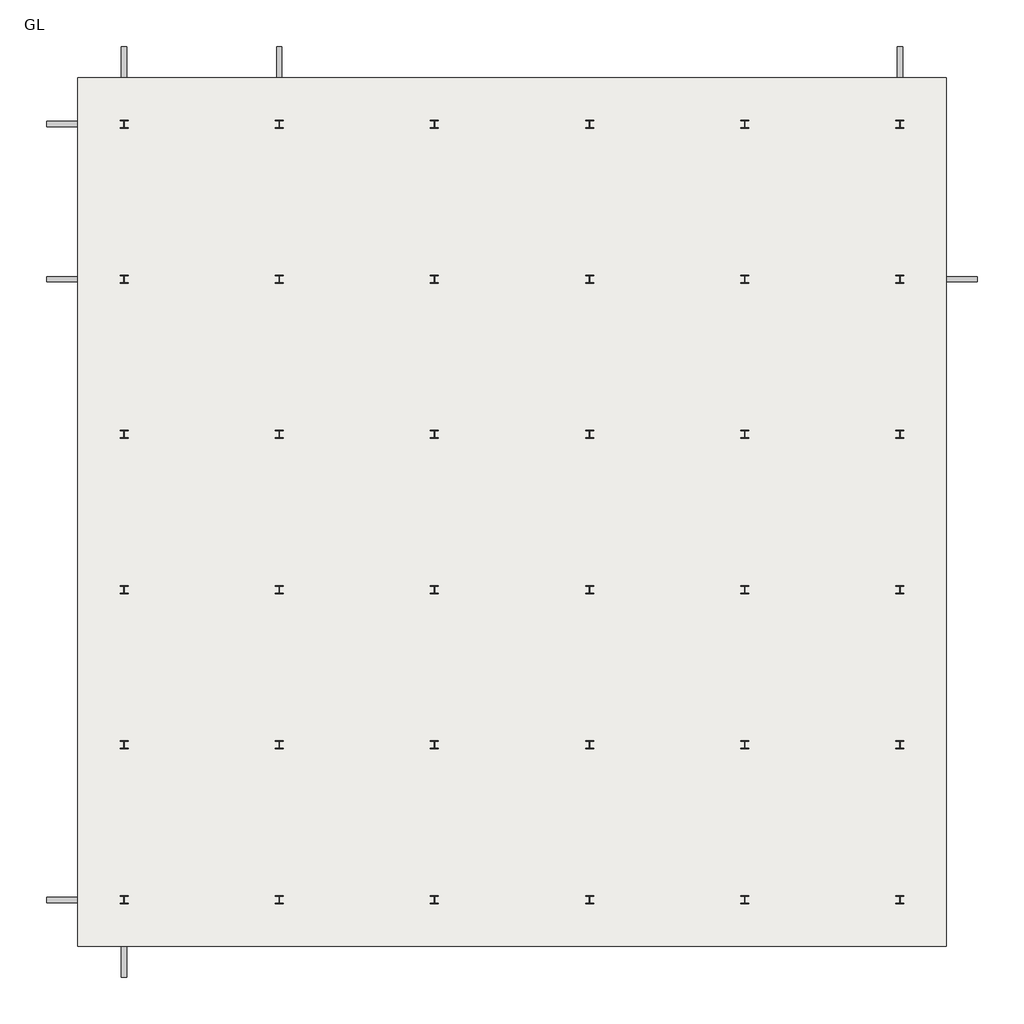
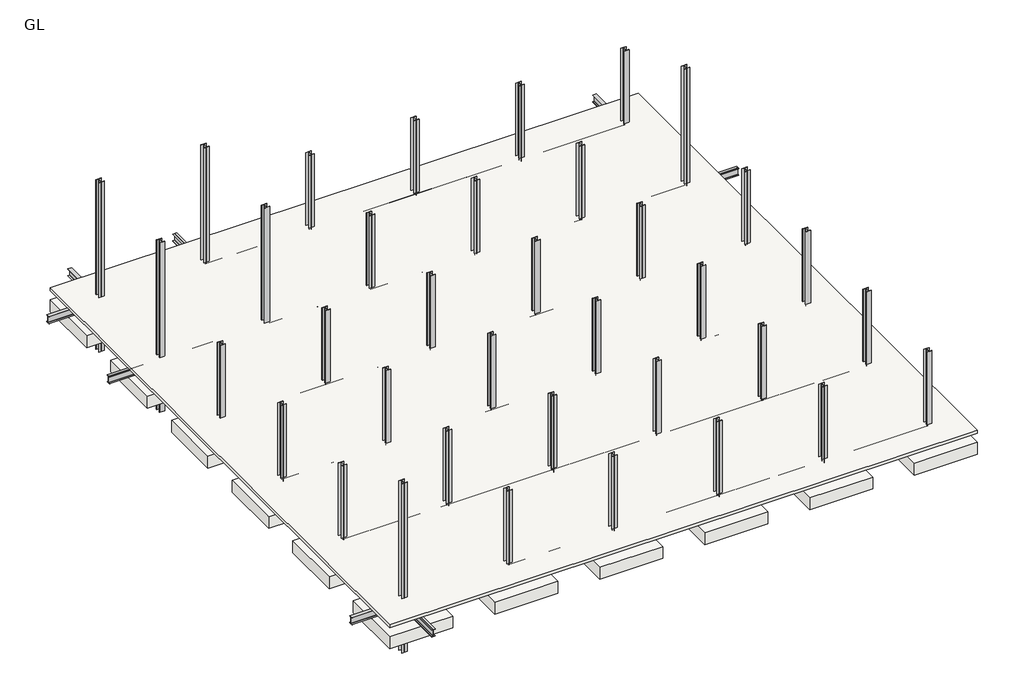
# One storey: 60 beams, 37 slabs, 36 columns.
"""IFC4 building model written with IfcOpenShell, lengths in millimetres."""

from ifc_helpers import new_model, si_unit, frame, origin, place, context, project, spatial, polyline, outline, extrude, transform, mapped, element, save
from components import w_shapes_w14x30_541e514d, w_shapes_w14x30_920474df, w_shapes_column_w10x49_053c6d64, w_shapes_column_w10x49_3bdde7d6, footing_rectangular_3mx3mx0_6m_b12d3fe5

model = new_model("IFC4")

# Units and contexts
model_context = context("Model", 3, world=origin())
ifc_project = project(units=[si_unit("LENGTHUNIT", "METRE", prefix="MILLI")], contexts=[model_context])

# Site, building, storey
site = spatial("IfcSite", under=ifc_project)
building = spatial("IfcBuilding", under=site)
storey = spatial("IfcBuildingStorey", under=building, Name="GL", Elevation=0.0)

# Beams
placement = place(None, origin())
w_shapes_w14x30_shape = w_shapes_w14x30_541e514d(model_context)
element("IfcBeam", 1, ObjectType="W Shapes : W14X30", at=placement, inside=storey, context=model_context, shape_type="MappedRepresentation", body=[
    mapped(w_shapes_w14x30_shape, transform((-15925.6378857, -5961.1374521, 281.94), x_axis=(1.0, 0.0, 0.0), y_axis=(0.0, 1.0, 0.0), z_axis=(0.0, 0.0, 1.0))),
])
element("IfcBeam", 2, ObjectType="W Shapes : W14X30", at=placement, inside=storey, context=model_context, shape_type="MappedRepresentation", body=[
    mapped(w_shapes_w14x30_shape, transform((-15925.6378857, 14038.8625479, 281.94), x_axis=(1.0, 0.0, 0.0), y_axis=(0.0, 1.0, 0.0), z_axis=(0.0, 0.0, 1.0))),
])
element("IfcBeam", 3, ObjectType="W Shapes : W14X30", at=placement, inside=storey, context=model_context, shape_type="MappedRepresentation", body=[
    mapped(w_shapes_w14x30_shape, transform((4074.3621143, 14038.8625479, 281.94), x_axis=(1.0, 0.0, 0.0), y_axis=(0.0, 1.0, 0.0), z_axis=(0.0, 0.0, 1.0))),
])
element("IfcBeam", 4, ObjectType="W Shapes : W14X30", at=placement, inside=storey, context=model_context, shape_type="MappedRepresentation", body=[
    mapped(w_shapes_w14x30_shape, transform((-15925.6378857, 19038.8625479, 281.94), x_axis=(1.0, 0.0, 0.0), y_axis=(0.0, 1.0, 0.0), z_axis=(0.0, 0.0, 1.0))),
])
element("IfcBeam", 5, ObjectType="W Shapes : W14X30", at=placement, inside=storey, context=model_context, shape_type="MappedRepresentation", body=[
    mapped(w_shapes_w14x30_shape, transform((6574.3621143, 11538.8625479, 281.94), x_axis=(0.0, 1.0, 0.0), y_axis=(-1.0, 0.0, 0.0), z_axis=(0.0, 0.0, 1.0))),
])
element("IfcBeam", 6, ObjectType="W Shapes : W14X30", at=placement, inside=storey, context=model_context, shape_type="MappedRepresentation", body=[
    mapped(w_shapes_w14x30_shape, transform((6574.3621143, 16538.8625479, 281.94), x_axis=(0.0, 1.0, 0.0), y_axis=(-1.0, 0.0, 0.0), z_axis=(0.0, 0.0, 1.0))),
])
element("IfcBeam", 7, ObjectType="W Shapes : W14X30", at=placement, inside=storey, context=model_context, shape_type="MappedRepresentation", body=[
    mapped(w_shapes_w14x30_shape, transform((-13425.6378857, 11538.8625479, 281.94), x_axis=(0.0, 1.0, 0.0), y_axis=(-1.0, 0.0, 0.0), z_axis=(0.0, 0.0, 1.0))),
])
element("IfcBeam", 8, ObjectType="W Shapes : W14X30", at=placement, inside=storey, context=model_context, shape_type="MappedRepresentation", body=[
    mapped(w_shapes_w14x30_shape, transform((-13425.6378857, 16538.8625479, 281.94), x_axis=(0.0, 1.0, 0.0), y_axis=(-1.0, 0.0, 0.0), z_axis=(0.0, 0.0, 1.0))),
])
element("IfcBeam", 9, ObjectType="W Shapes : W14X30", at=placement, inside=storey, context=model_context, shape_type="MappedRepresentation", body=[
    mapped(w_shapes_w14x30_shape, transform((-18425.6378857, -3461.1374521, 281.94), x_axis=(0.0, 1.0, 0.0), y_axis=(-1.0, 0.0, 0.0), z_axis=(0.0, 0.0, 1.0))),
])
element("IfcBeam", 10, ObjectType="W Shapes : W14X30", at=placement, inside=storey, context=model_context, shape_type="MappedRepresentation", body=[
    mapped(w_shapes_w14x30_shape, transform((-18425.6378857, 16538.8625479, 281.94), x_axis=(0.0, 1.0, 0.0), y_axis=(-1.0, 0.0, 0.0), z_axis=(0.0, 0.0, 1.0))),
])
element("IfcBeam", 11, ObjectType="W Shapes : W14X30", at=placement, inside=storey, context=model_context, shape_type="MappedRepresentation", body=[
    mapped(w_shapes_w14x30_shape, transform((-10925.6378857, 14038.8625479, 281.94), x_axis=(1.0, 0.0, 0.0), y_axis=(0.0, 1.0, 0.0), z_axis=(0.0, 0.0, 1.0))),
])
w_shapes_w14x30_2_shape = w_shapes_w14x30_920474df(model_context)
element("IfcBeam", 12, ObjectType="W Shapes : W14X30", at=placement, inside=storey, context=model_context, shape_type="MappedRepresentation", body=[
    mapped(w_shapes_w14x30_2_shape, transform((-10925.6378857, -5961.1374521, 281.94), x_axis=(1.0, 0.0, 0.0), y_axis=(0.0, 1.0, 0.0), z_axis=(0.0, 0.0, 1.0))),
])
element("IfcBeam", 13, ObjectType="W Shapes : W14X30", at=placement, inside=storey, context=model_context, shape_type="MappedRepresentation", body=[
    mapped(w_shapes_w14x30_2_shape, transform((-5925.6378857, -5961.1374521, 281.94), x_axis=(1.0, 0.0, 0.0), y_axis=(0.0, 1.0, 0.0), z_axis=(0.0, 0.0, 1.0))),
])
element("IfcBeam", 14, ObjectType="W Shapes : W14X30", at=placement, inside=storey, context=model_context, shape_type="MappedRepresentation", body=[
    mapped(w_shapes_w14x30_2_shape, transform((-925.6378857, -5961.1374521, 281.94), x_axis=(1.0, 0.0, 0.0), y_axis=(0.0, 1.0, 0.0), z_axis=(0.0, 0.0, 1.0))),
])
element("IfcBeam", 15, ObjectType="W Shapes : W14X30", at=placement, inside=storey, context=model_context, shape_type="MappedRepresentation", body=[
    mapped(w_shapes_w14x30_2_shape, transform((4074.3621143, -5961.1374521, 281.94), x_axis=(1.0, 0.0, 0.0), y_axis=(0.0, 1.0, 0.0), z_axis=(0.0, 0.0, 1.0))),
])
element("IfcBeam", 16, ObjectType="W Shapes : W14X30", at=placement, inside=storey, context=model_context, shape_type="MappedRepresentation", body=[
    mapped(w_shapes_w14x30_2_shape, transform((-15925.6378857, -961.1374521, 281.94), x_axis=(1.0, 0.0, 0.0), y_axis=(0.0, 1.0, 0.0), z_axis=(0.0, 0.0, 1.0))),
])
element("IfcBeam", 17, ObjectType="W Shapes : W14X30", at=placement, inside=storey, context=model_context, shape_type="MappedRepresentation", body=[
    mapped(w_shapes_w14x30_2_shape, transform((-10925.6378857, -961.1374521, 281.94), x_axis=(1.0, 0.0, 0.0), y_axis=(0.0, 1.0, 0.0), z_axis=(0.0, 0.0, 1.0))),
])
element("IfcBeam", 18, ObjectType="W Shapes : W14X30", at=placement, inside=storey, context=model_context, shape_type="MappedRepresentation", body=[
    mapped(w_shapes_w14x30_2_shape, transform((-5925.6378857, -961.1374521, 281.94), x_axis=(1.0, 0.0, 0.0), y_axis=(0.0, 1.0, 0.0), z_axis=(0.0, 0.0, 1.0))),
])
element("IfcBeam", 19, ObjectType="W Shapes : W14X30", at=placement, inside=storey, context=model_context, shape_type="MappedRepresentation", body=[
    mapped(w_shapes_w14x30_2_shape, transform((-925.6378857, -961.1374521, 281.94), x_axis=(1.0, 0.0, 0.0), y_axis=(0.0, 1.0, 0.0), z_axis=(0.0, 0.0, 1.0))),
])
element("IfcBeam", 20, ObjectType="W Shapes : W14X30", at=placement, inside=storey, context=model_context, shape_type="MappedRepresentation", body=[
    mapped(w_shapes_w14x30_2_shape, transform((4074.3621143, -961.1374521, 281.94), x_axis=(1.0, 0.0, 0.0), y_axis=(0.0, 1.0, 0.0), z_axis=(0.0, 0.0, 1.0))),
])
element("IfcBeam", 21, ObjectType="W Shapes : W14X30", at=placement, inside=storey, context=model_context, shape_type="MappedRepresentation", body=[
    mapped(w_shapes_w14x30_2_shape, transform((-15925.6378857, 4038.8625479, 281.94), x_axis=(1.0, 0.0, 0.0), y_axis=(0.0, 1.0, 0.0), z_axis=(0.0, 0.0, 1.0))),
])
element("IfcBeam", 22, ObjectType="W Shapes : W14X30", at=placement, inside=storey, context=model_context, shape_type="MappedRepresentation", body=[
    mapped(w_shapes_w14x30_2_shape, transform((-10925.6378857, 4038.8625479, 281.94), x_axis=(1.0, 0.0, 0.0), y_axis=(0.0, 1.0, 0.0), z_axis=(0.0, 0.0, 1.0))),
])
element("IfcBeam", 23, ObjectType="W Shapes : W14X30", at=placement, inside=storey, context=model_context, shape_type="MappedRepresentation", body=[
    mapped(w_shapes_w14x30_2_shape, transform((-5925.6378857, 4038.8625479, 281.94), x_axis=(1.0, 0.0, 0.0), y_axis=(0.0, 1.0, 0.0), z_axis=(0.0, 0.0, 1.0))),
])
element("IfcBeam", 24, ObjectType="W Shapes : W14X30", at=placement, inside=storey, context=model_context, shape_type="MappedRepresentation", body=[
    mapped(w_shapes_w14x30_2_shape, transform((-925.6378857, 4038.8625479, 281.94), x_axis=(1.0, 0.0, 0.0), y_axis=(0.0, 1.0, 0.0), z_axis=(0.0, 0.0, 1.0))),
])
element("IfcBeam", 25, ObjectType="W Shapes : W14X30", at=placement, inside=storey, context=model_context, shape_type="MappedRepresentation", body=[
    mapped(w_shapes_w14x30_2_shape, transform((4074.3621143, 4038.8625479, 281.94), x_axis=(1.0, 0.0, 0.0), y_axis=(0.0, 1.0, 0.0), z_axis=(0.0, 0.0, 1.0))),
])
element("IfcBeam", 26, ObjectType="W Shapes : W14X30", at=placement, inside=storey, context=model_context, shape_type="MappedRepresentation", body=[
    mapped(w_shapes_w14x30_2_shape, transform((-15925.6378857, 9038.8625479, 281.94), x_axis=(1.0, 0.0, 0.0), y_axis=(0.0, 1.0, 0.0), z_axis=(0.0, 0.0, 1.0))),
])
element("IfcBeam", 27, ObjectType="W Shapes : W14X30", at=placement, inside=storey, context=model_context, shape_type="MappedRepresentation", body=[
    mapped(w_shapes_w14x30_2_shape, transform((-10925.6378857, 9038.8625479, 281.94), x_axis=(1.0, 0.0, 0.0), y_axis=(0.0, 1.0, 0.0), z_axis=(0.0, 0.0, 1.0))),
])
element("IfcBeam", 28, ObjectType="W Shapes : W14X30", at=placement, inside=storey, context=model_context, shape_type="MappedRepresentation", body=[
    mapped(w_shapes_w14x30_2_shape, transform((-5925.6378857, 9038.8625479, 281.94), x_axis=(1.0, 0.0, 0.0), y_axis=(0.0, 1.0, 0.0), z_axis=(0.0, 0.0, 1.0))),
])
element("IfcBeam", 29, ObjectType="W Shapes : W14X30", at=placement, inside=storey, context=model_context, shape_type="MappedRepresentation", body=[
    mapped(w_shapes_w14x30_2_shape, transform((-925.6378857, 9038.8625479, 281.94), x_axis=(1.0, 0.0, 0.0), y_axis=(0.0, 1.0, 0.0), z_axis=(0.0, 0.0, 1.0))),
])
element("IfcBeam", 30, ObjectType="W Shapes : W14X30", at=placement, inside=storey, context=model_context, shape_type="MappedRepresentation", body=[
    mapped(w_shapes_w14x30_2_shape, transform((4074.3621143, 9038.8625479, 281.94), x_axis=(1.0, 0.0, 0.0), y_axis=(0.0, 1.0, 0.0), z_axis=(0.0, 0.0, 1.0))),
])
element("IfcBeam", 31, ObjectType="W Shapes : W14X30", at=placement, inside=storey, context=model_context, shape_type="MappedRepresentation", body=[
    mapped(w_shapes_w14x30_2_shape, transform((-5925.6378857, 14038.8625479, 281.94), x_axis=(1.0, 0.0, 0.0), y_axis=(0.0, 1.0, 0.0), z_axis=(0.0, 0.0, 1.0))),
])
element("IfcBeam", 32, ObjectType="W Shapes : W14X30", at=placement, inside=storey, context=model_context, shape_type="MappedRepresentation", body=[
    mapped(w_shapes_w14x30_2_shape, transform((-925.6378857, 14038.8625479, 281.94), x_axis=(1.0, 0.0, 0.0), y_axis=(0.0, 1.0, 0.0), z_axis=(0.0, 0.0, 1.0))),
])
element("IfcBeam", 33, ObjectType="W Shapes : W14X30", at=placement, inside=storey, context=model_context, shape_type="MappedRepresentation", body=[
    mapped(w_shapes_w14x30_2_shape, transform((-10925.6378857, 19038.8625479, 281.94), x_axis=(1.0, 0.0, 0.0), y_axis=(0.0, 1.0, 0.0), z_axis=(0.0, 0.0, 1.0))),
])
element("IfcBeam", 34, ObjectType="W Shapes : W14X30", at=placement, inside=storey, context=model_context, shape_type="MappedRepresentation", body=[
    mapped(w_shapes_w14x30_2_shape, transform((-5925.6378857, 19038.8625479, 281.94), x_axis=(1.0, 0.0, 0.0), y_axis=(0.0, 1.0, 0.0), z_axis=(0.0, 0.0, 1.0))),
])
element("IfcBeam", 35, ObjectType="W Shapes : W14X30", at=placement, inside=storey, context=model_context, shape_type="MappedRepresentation", body=[
    mapped(w_shapes_w14x30_2_shape, transform((-925.6378857, 19038.8625479, 281.94), x_axis=(1.0, 0.0, 0.0), y_axis=(0.0, 1.0, 0.0), z_axis=(0.0, 0.0, 1.0))),
])
element("IfcBeam", 36, ObjectType="W Shapes : W14X30", at=placement, inside=storey, context=model_context, shape_type="MappedRepresentation", body=[
    mapped(w_shapes_w14x30_2_shape, transform((4074.3621143, 19038.8625479, 281.94), x_axis=(1.0, 0.0, 0.0), y_axis=(0.0, 1.0, 0.0), z_axis=(0.0, 0.0, 1.0))),
])
element("IfcBeam", 37, ObjectType="W Shapes : W14X30", at=placement, inside=storey, context=model_context, shape_type="MappedRepresentation", body=[
    mapped(w_shapes_w14x30_2_shape, transform((6574.3621143, -3461.1374521, 281.94), x_axis=(0.0, 1.0, 0.0), y_axis=(-1.0, 0.0, 0.0), z_axis=(0.0, 0.0, 1.0))),
])
element("IfcBeam", 38, ObjectType="W Shapes : W14X30", at=placement, inside=storey, context=model_context, shape_type="MappedRepresentation", body=[
    mapped(w_shapes_w14x30_2_shape, transform((6574.3621143, 1538.8625479, 281.94), x_axis=(0.0, 1.0, 0.0), y_axis=(-1.0, 0.0, 0.0), z_axis=(0.0, 0.0, 1.0))),
])
element("IfcBeam", 39, ObjectType="W Shapes : W14X30", at=placement, inside=storey, context=model_context, shape_type="MappedRepresentation", body=[
    mapped(w_shapes_w14x30_2_shape, transform((6574.3621143, 6538.8625479, 281.94), x_axis=(0.0, 1.0, 0.0), y_axis=(-1.0, 0.0, 0.0), z_axis=(0.0, 0.0, 1.0))),
])
element("IfcBeam", 40, ObjectType="W Shapes : W14X30", at=placement, inside=storey, context=model_context, shape_type="MappedRepresentation", body=[
    mapped(w_shapes_w14x30_2_shape, transform((1574.3621143, -3461.1374521, 281.94), x_axis=(0.0, 1.0, 0.0), y_axis=(-1.0, 0.0, 0.0), z_axis=(0.0, 0.0, 1.0))),
])
element("IfcBeam", 41, ObjectType="W Shapes : W14X30", at=placement, inside=storey, context=model_context, shape_type="MappedRepresentation", body=[
    mapped(w_shapes_w14x30_2_shape, transform((1574.3621143, 1538.8625479, 281.94), x_axis=(0.0, 1.0, 0.0), y_axis=(-1.0, 0.0, 0.0), z_axis=(0.0, 0.0, 1.0))),
])
element("IfcBeam", 42, ObjectType="W Shapes : W14X30", at=placement, inside=storey, context=model_context, shape_type="MappedRepresentation", body=[
    mapped(w_shapes_w14x30_2_shape, transform((1574.3621143, 6538.8625479, 281.94), x_axis=(0.0, 1.0, 0.0), y_axis=(-1.0, 0.0, 0.0), z_axis=(0.0, 0.0, 1.0))),
])
element("IfcBeam", 43, ObjectType="W Shapes : W14X30", at=placement, inside=storey, context=model_context, shape_type="MappedRepresentation", body=[
    mapped(w_shapes_w14x30_2_shape, transform((1574.3621143, 11538.8625479, 281.94), x_axis=(0.0, 1.0, 0.0), y_axis=(-1.0, 0.0, 0.0), z_axis=(0.0, 0.0, 1.0))),
])
element("IfcBeam", 44, ObjectType="W Shapes : W14X30", at=placement, inside=storey, context=model_context, shape_type="MappedRepresentation", body=[
    mapped(w_shapes_w14x30_2_shape, transform((1574.3621143, 16538.8625479, 281.94), x_axis=(0.0, 1.0, 0.0), y_axis=(-1.0, 0.0, 0.0), z_axis=(0.0, 0.0, 1.0))),
])
element("IfcBeam", 45, ObjectType="W Shapes : W14X30", at=placement, inside=storey, context=model_context, shape_type="MappedRepresentation", body=[
    mapped(w_shapes_w14x30_2_shape, transform((-3425.6378857, -3461.1374521, 281.94), x_axis=(0.0, 1.0, 0.0), y_axis=(-1.0, 0.0, 0.0), z_axis=(0.0, 0.0, 1.0))),
])
element("IfcBeam", 46, ObjectType="W Shapes : W14X30", at=placement, inside=storey, context=model_context, shape_type="MappedRepresentation", body=[
    mapped(w_shapes_w14x30_2_shape, transform((-3425.6378857, 1538.8625479, 281.94), x_axis=(0.0, 1.0, 0.0), y_axis=(-1.0, 0.0, 0.0), z_axis=(0.0, 0.0, 1.0))),
])
element("IfcBeam", 47, ObjectType="W Shapes : W14X30", at=placement, inside=storey, context=model_context, shape_type="MappedRepresentation", body=[
    mapped(w_shapes_w14x30_2_shape, transform((-3425.6378857, 6538.8625479, 281.94), x_axis=(0.0, 1.0, 0.0), y_axis=(-1.0, 0.0, 0.0), z_axis=(0.0, 0.0, 1.0))),
])
element("IfcBeam", 48, ObjectType="W Shapes : W14X30", at=placement, inside=storey, context=model_context, shape_type="MappedRepresentation", body=[
    mapped(w_shapes_w14x30_2_shape, transform((-3425.6378857, 11538.8625479, 281.94), x_axis=(0.0, 1.0, 0.0), y_axis=(-1.0, 0.0, 0.0), z_axis=(0.0, 0.0, 1.0))),
])
element("IfcBeam", 49, ObjectType="W Shapes : W14X30", at=placement, inside=storey, context=model_context, shape_type="MappedRepresentation", body=[
    mapped(w_shapes_w14x30_2_shape, transform((-3425.6378857, 16538.8625479, 281.94), x_axis=(0.0, 1.0, 0.0), y_axis=(-1.0, 0.0, 0.0), z_axis=(0.0, 0.0, 1.0))),
])
element("IfcBeam", 50, ObjectType="W Shapes : W14X30", at=placement, inside=storey, context=model_context, shape_type="MappedRepresentation", body=[
    mapped(w_shapes_w14x30_2_shape, transform((-8425.6378857, -3461.1374521, 281.94), x_axis=(0.0, 1.0, 0.0), y_axis=(-1.0, 0.0, 0.0), z_axis=(0.0, 0.0, 1.0))),
])
element("IfcBeam", 51, ObjectType="W Shapes : W14X30", at=placement, inside=storey, context=model_context, shape_type="MappedRepresentation", body=[
    mapped(w_shapes_w14x30_2_shape, transform((-8425.6378857, 1538.8625479, 281.94), x_axis=(0.0, 1.0, 0.0), y_axis=(-1.0, 0.0, 0.0), z_axis=(0.0, 0.0, 1.0))),
])
element("IfcBeam", 52, ObjectType="W Shapes : W14X30", at=placement, inside=storey, context=model_context, shape_type="MappedRepresentation", body=[
    mapped(w_shapes_w14x30_2_shape, transform((-8425.6378857, 6538.8625479, 281.94), x_axis=(0.0, 1.0, 0.0), y_axis=(-1.0, 0.0, 0.0), z_axis=(0.0, 0.0, 1.0))),
])
element("IfcBeam", 53, ObjectType="W Shapes : W14X30", at=placement, inside=storey, context=model_context, shape_type="MappedRepresentation", body=[
    mapped(w_shapes_w14x30_2_shape, transform((-8425.6378857, 11538.8625479, 281.94), x_axis=(0.0, 1.0, 0.0), y_axis=(-1.0, 0.0, 0.0), z_axis=(0.0, 0.0, 1.0))),
])
element("IfcBeam", 54, ObjectType="W Shapes : W14X30", at=placement, inside=storey, context=model_context, shape_type="MappedRepresentation", body=[
    mapped(w_shapes_w14x30_2_shape, transform((-8425.6378857, 16538.8625479, 281.94), x_axis=(0.0, 1.0, 0.0), y_axis=(-1.0, 0.0, 0.0), z_axis=(0.0, 0.0, 1.0))),
])
element("IfcBeam", 55, ObjectType="W Shapes : W14X30", at=placement, inside=storey, context=model_context, shape_type="MappedRepresentation", body=[
    mapped(w_shapes_w14x30_2_shape, transform((-13425.6378857, -3461.1374521, 281.94), x_axis=(0.0, 1.0, 0.0), y_axis=(-1.0, 0.0, 0.0), z_axis=(0.0, 0.0, 1.0))),
])
element("IfcBeam", 56, ObjectType="W Shapes : W14X30", at=placement, inside=storey, context=model_context, shape_type="MappedRepresentation", body=[
    mapped(w_shapes_w14x30_2_shape, transform((-13425.6378857, 1538.8625479, 281.94), x_axis=(0.0, 1.0, 0.0), y_axis=(-1.0, 0.0, 0.0), z_axis=(0.0, 0.0, 1.0))),
])
element("IfcBeam", 57, ObjectType="W Shapes : W14X30", at=placement, inside=storey, context=model_context, shape_type="MappedRepresentation", body=[
    mapped(w_shapes_w14x30_2_shape, transform((-13425.6378857, 6538.8625479, 281.94), x_axis=(0.0, 1.0, 0.0), y_axis=(-1.0, 0.0, 0.0), z_axis=(0.0, 0.0, 1.0))),
])
element("IfcBeam", 58, ObjectType="W Shapes : W14X30", at=placement, inside=storey, context=model_context, shape_type="MappedRepresentation", body=[
    mapped(w_shapes_w14x30_2_shape, transform((-18425.6378857, 1538.8625479, 281.94), x_axis=(0.0, 1.0, 0.0), y_axis=(-1.0, 0.0, 0.0), z_axis=(0.0, 0.0, 1.0))),
])
element("IfcBeam", 59, ObjectType="W Shapes : W14X30", at=placement, inside=storey, context=model_context, shape_type="MappedRepresentation", body=[
    mapped(w_shapes_w14x30_2_shape, transform((-18425.6378857, 6538.8625479, 281.94), x_axis=(0.0, 1.0, 0.0), y_axis=(-1.0, 0.0, 0.0), z_axis=(0.0, 0.0, 1.0))),
])
element("IfcBeam", 60, ObjectType="W Shapes : W14X30", at=placement, inside=storey, context=model_context, shape_type="MappedRepresentation", body=[
    mapped(w_shapes_w14x30_2_shape, transform((-18425.6378857, 11538.8625479, 281.94), x_axis=(0.0, 1.0, 0.0), y_axis=(-1.0, 0.0, 0.0), z_axis=(0.0, 0.0, 1.0))),
])

# Columns
w_shapes_column_w10x49_shape = w_shapes_column_w10x49_053c6d64(model_context)
element("IfcColumn", 61, ObjectType="W Shapes-Column : W10X49", at=placement, inside=storey, context=model_context, shape_type="MappedRepresentation", body=[
    mapped(w_shapes_column_w10x49_shape, transform((6574.3621143, -5961.1374521, 0.0), x_axis=(1.0, 0.0, 0.0), y_axis=(0.0, 1.0, 0.0), z_axis=(0.0, 0.0, 1.0))),
])
element("IfcColumn", 62, ObjectType="W Shapes-Column : W10X49", at=placement, inside=storey, context=model_context, shape_type="MappedRepresentation", body=[
    mapped(w_shapes_column_w10x49_shape, transform((1574.3621143, -5961.1374521, 0.0), x_axis=(1.0, 0.0, 0.0), y_axis=(0.0, 1.0, 0.0), z_axis=(0.0, 0.0, 1.0))),
])
element("IfcColumn", 63, ObjectType="W Shapes-Column : W10X49", at=placement, inside=storey, context=model_context, shape_type="MappedRepresentation", body=[
    mapped(w_shapes_column_w10x49_shape, transform((-3425.6378857, -5961.1374521, 0.0), x_axis=(1.0, 0.0, 0.0), y_axis=(0.0, 1.0, 0.0), z_axis=(0.0, 0.0, 1.0))),
])
element("IfcColumn", 64, ObjectType="W Shapes-Column : W10X49", at=placement, inside=storey, context=model_context, shape_type="MappedRepresentation", body=[
    mapped(w_shapes_column_w10x49_shape, transform((-8425.6378857, -5961.1374521, 0.0), x_axis=(1.0, 0.0, 0.0), y_axis=(0.0, 1.0, 0.0), z_axis=(0.0, 0.0, 1.0))),
])
element("IfcColumn", 65, ObjectType="W Shapes-Column : W10X49", at=placement, inside=storey, context=model_context, shape_type="MappedRepresentation", body=[
    mapped(w_shapes_column_w10x49_shape, transform((-13425.6378857, -5961.1374521, 0.0), x_axis=(1.0, 0.0, 0.0), y_axis=(0.0, 1.0, 0.0), z_axis=(0.0, 0.0, 1.0))),
])
element("IfcColumn", 66, ObjectType="W Shapes-Column : W10X49", at=placement, inside=storey, context=model_context, shape_type="MappedRepresentation", body=[
    mapped(w_shapes_column_w10x49_shape, transform((6574.3621143, -961.1374521, 0.0), x_axis=(1.0, 0.0, 0.0), y_axis=(0.0, 1.0, 0.0), z_axis=(0.0, 0.0, 1.0))),
])
element("IfcColumn", 67, ObjectType="W Shapes-Column : W10X49", at=placement, inside=storey, context=model_context, shape_type="MappedRepresentation", body=[
    mapped(w_shapes_column_w10x49_shape, transform((1574.3621143, -961.1374521, 0.0), x_axis=(1.0, 0.0, 0.0), y_axis=(0.0, 1.0, 0.0), z_axis=(0.0, 0.0, 1.0))),
])
element("IfcColumn", 68, ObjectType="W Shapes-Column : W10X49", at=placement, inside=storey, context=model_context, shape_type="MappedRepresentation", body=[
    mapped(w_shapes_column_w10x49_shape, transform((-3425.6378857, -961.1374521, 0.0), x_axis=(1.0, 0.0, 0.0), y_axis=(0.0, 1.0, 0.0), z_axis=(0.0, 0.0, 1.0))),
])
element("IfcColumn", 69, ObjectType="W Shapes-Column : W10X49", at=placement, inside=storey, context=model_context, shape_type="MappedRepresentation", body=[
    mapped(w_shapes_column_w10x49_shape, transform((-8425.6378857, -961.1374521, 0.0), x_axis=(1.0, 0.0, 0.0), y_axis=(0.0, 1.0, 0.0), z_axis=(0.0, 0.0, 1.0))),
])
element("IfcColumn", 70, ObjectType="W Shapes-Column : W10X49", at=placement, inside=storey, context=model_context, shape_type="MappedRepresentation", body=[
    mapped(w_shapes_column_w10x49_shape, transform((-13425.6378857, -961.1374521, 0.0), x_axis=(1.0, 0.0, 0.0), y_axis=(0.0, 1.0, 0.0), z_axis=(0.0, 0.0, 1.0))),
])
element("IfcColumn", 71, ObjectType="W Shapes-Column : W10X49", at=placement, inside=storey, context=model_context, shape_type="MappedRepresentation", body=[
    mapped(w_shapes_column_w10x49_shape, transform((-18425.6378857, -961.1374521, 0.0), x_axis=(1.0, 0.0, 0.0), y_axis=(0.0, 1.0, 0.0), z_axis=(0.0, 0.0, 1.0))),
])
element("IfcColumn", 72, ObjectType="W Shapes-Column : W10X49", at=placement, inside=storey, context=model_context, shape_type="MappedRepresentation", body=[
    mapped(w_shapes_column_w10x49_shape, transform((6574.3621143, 4038.8625479, 0.0), x_axis=(1.0, 0.0, 0.0), y_axis=(0.0, 1.0, 0.0), z_axis=(0.0, 0.0, 1.0))),
])
element("IfcColumn", 73, ObjectType="W Shapes-Column : W10X49", at=placement, inside=storey, context=model_context, shape_type="MappedRepresentation", body=[
    mapped(w_shapes_column_w10x49_shape, transform((1574.3621143, 4038.8625479, 0.0), x_axis=(1.0, 0.0, 0.0), y_axis=(0.0, 1.0, 0.0), z_axis=(0.0, 0.0, 1.0))),
])
element("IfcColumn", 74, ObjectType="W Shapes-Column : W10X49", at=placement, inside=storey, context=model_context, shape_type="MappedRepresentation", body=[
    mapped(w_shapes_column_w10x49_shape, transform((-3425.6378857, 4038.8625479, 0.0), x_axis=(1.0, 0.0, 0.0), y_axis=(0.0, 1.0, 0.0), z_axis=(0.0, 0.0, 1.0))),
])
element("IfcColumn", 75, ObjectType="W Shapes-Column : W10X49", at=placement, inside=storey, context=model_context, shape_type="MappedRepresentation", body=[
    mapped(w_shapes_column_w10x49_shape, transform((-8425.6378857, 4038.8625479, 0.0), x_axis=(1.0, 0.0, 0.0), y_axis=(0.0, 1.0, 0.0), z_axis=(0.0, 0.0, 1.0))),
])
element("IfcColumn", 76, ObjectType="W Shapes-Column : W10X49", at=placement, inside=storey, context=model_context, shape_type="MappedRepresentation", body=[
    mapped(w_shapes_column_w10x49_shape, transform((-13425.6378857, 4038.8625479, 0.0), x_axis=(1.0, 0.0, 0.0), y_axis=(0.0, 1.0, 0.0), z_axis=(0.0, 0.0, 1.0))),
])
element("IfcColumn", 77, ObjectType="W Shapes-Column : W10X49", at=placement, inside=storey, context=model_context, shape_type="MappedRepresentation", body=[
    mapped(w_shapes_column_w10x49_shape, transform((-18425.6378857, 4038.8625479, 0.0), x_axis=(1.0, 0.0, 0.0), y_axis=(0.0, 1.0, 0.0), z_axis=(0.0, 0.0, 1.0))),
])
element("IfcColumn", 78, ObjectType="W Shapes-Column : W10X49", at=placement, inside=storey, context=model_context, shape_type="MappedRepresentation", body=[
    mapped(w_shapes_column_w10x49_shape, transform((6574.3621143, 9038.8625479, 0.0), x_axis=(1.0, 0.0, 0.0), y_axis=(0.0, 1.0, 0.0), z_axis=(0.0, 0.0, 1.0))),
])
element("IfcColumn", 79, ObjectType="W Shapes-Column : W10X49", at=placement, inside=storey, context=model_context, shape_type="MappedRepresentation", body=[
    mapped(w_shapes_column_w10x49_shape, transform((1574.3621143, 9038.8625479, 0.0), x_axis=(1.0, 0.0, 0.0), y_axis=(0.0, 1.0, 0.0), z_axis=(0.0, 0.0, 1.0))),
])
element("IfcColumn", 80, ObjectType="W Shapes-Column : W10X49", at=placement, inside=storey, context=model_context, shape_type="MappedRepresentation", body=[
    mapped(w_shapes_column_w10x49_shape, transform((-3425.6378857, 9038.8625479, 0.0), x_axis=(1.0, 0.0, 0.0), y_axis=(0.0, 1.0, 0.0), z_axis=(0.0, 0.0, 1.0))),
])
element("IfcColumn", 81, ObjectType="W Shapes-Column : W10X49", at=placement, inside=storey, context=model_context, shape_type="MappedRepresentation", body=[
    mapped(w_shapes_column_w10x49_shape, transform((-8425.6378857, 9038.8625479, 0.0), x_axis=(1.0, 0.0, 0.0), y_axis=(0.0, 1.0, 0.0), z_axis=(0.0, 0.0, 1.0))),
])
element("IfcColumn", 82, ObjectType="W Shapes-Column : W10X49", at=placement, inside=storey, context=model_context, shape_type="MappedRepresentation", body=[
    mapped(w_shapes_column_w10x49_shape, transform((-13425.6378857, 9038.8625479, 0.0), x_axis=(1.0, 0.0, 0.0), y_axis=(0.0, 1.0, 0.0), z_axis=(0.0, 0.0, 1.0))),
])
element("IfcColumn", 83, ObjectType="W Shapes-Column : W10X49", at=placement, inside=storey, context=model_context, shape_type="MappedRepresentation", body=[
    mapped(w_shapes_column_w10x49_shape, transform((-18425.6378857, 9038.8625479, 0.0), x_axis=(1.0, 0.0, 0.0), y_axis=(0.0, 1.0, 0.0), z_axis=(0.0, 0.0, 1.0))),
])
element("IfcColumn", 84, ObjectType="W Shapes-Column : W10X49", at=placement, inside=storey, context=model_context, shape_type="MappedRepresentation", body=[
    mapped(w_shapes_column_w10x49_shape, transform((1574.3621143, 14038.8625479, 0.0), x_axis=(1.0, 0.0, 0.0), y_axis=(0.0, 1.0, 0.0), z_axis=(0.0, 0.0, 1.0))),
])
element("IfcColumn", 85, ObjectType="W Shapes-Column : W10X49", at=placement, inside=storey, context=model_context, shape_type="MappedRepresentation", body=[
    mapped(w_shapes_column_w10x49_shape, transform((-3425.6378857, 14038.8625479, 0.0), x_axis=(1.0, 0.0, 0.0), y_axis=(0.0, 1.0, 0.0), z_axis=(0.0, 0.0, 1.0))),
])
element("IfcColumn", 86, ObjectType="W Shapes-Column : W10X49", at=placement, inside=storey, context=model_context, shape_type="MappedRepresentation", body=[
    mapped(w_shapes_column_w10x49_shape, transform((-8425.6378857, 14038.8625479, 0.0), x_axis=(1.0, 0.0, 0.0), y_axis=(0.0, 1.0, 0.0), z_axis=(0.0, 0.0, 1.0))),
])
element("IfcColumn", 87, ObjectType="W Shapes-Column : W10X49", at=placement, inside=storey, context=model_context, shape_type="MappedRepresentation", body=[
    mapped(w_shapes_column_w10x49_shape, transform((6574.3621143, 19038.8625479, 0.0), x_axis=(1.0, 0.0, 0.0), y_axis=(0.0, 1.0, 0.0), z_axis=(0.0, 0.0, 1.0))),
])
element("IfcColumn", 88, ObjectType="W Shapes-Column : W10X49", at=placement, inside=storey, context=model_context, shape_type="MappedRepresentation", body=[
    mapped(w_shapes_column_w10x49_shape, transform((1574.3621143, 19038.8625479, 0.0), x_axis=(1.0, 0.0, 0.0), y_axis=(0.0, 1.0, 0.0), z_axis=(0.0, 0.0, 1.0))),
])
element("IfcColumn", 89, ObjectType="W Shapes-Column : W10X49", at=placement, inside=storey, context=model_context, shape_type="MappedRepresentation", body=[
    mapped(w_shapes_column_w10x49_shape, transform((-3425.6378857, 19038.8625479, 0.0), x_axis=(1.0, 0.0, 0.0), y_axis=(0.0, 1.0, 0.0), z_axis=(0.0, 0.0, 1.0))),
])
element("IfcColumn", 90, ObjectType="W Shapes-Column : W10X49", at=placement, inside=storey, context=model_context, shape_type="MappedRepresentation", body=[
    mapped(w_shapes_column_w10x49_shape, transform((-8425.6378857, 19038.8625479, 0.0), x_axis=(1.0, 0.0, 0.0), y_axis=(0.0, 1.0, 0.0), z_axis=(0.0, 0.0, 1.0))),
])
w_shapes_column_w10x49_2_shape = w_shapes_column_w10x49_3bdde7d6(model_context)
element("IfcColumn", 91, ObjectType="W Shapes-Column : W10X49", at=placement, inside=storey, context=model_context, shape_type="MappedRepresentation", body=[
    mapped(w_shapes_column_w10x49_2_shape, transform((-18425.6378857, -5961.1374521, 0.0), x_axis=(1.0, 0.0, 0.0), y_axis=(0.0, 1.0, 0.0), z_axis=(0.0, 0.0, 1.0))),
])
element("IfcColumn", 92, ObjectType="W Shapes-Column : W10X49", at=placement, inside=storey, context=model_context, shape_type="MappedRepresentation", body=[
    mapped(w_shapes_column_w10x49_2_shape, transform((6574.3621143, 14038.8625479, 0.0), x_axis=(1.0, 0.0, 0.0), y_axis=(0.0, 1.0, 0.0), z_axis=(0.0, 0.0, 1.0))),
])
element("IfcColumn", 93, ObjectType="W Shapes-Column : W10X49", at=placement, inside=storey, context=model_context, shape_type="MappedRepresentation", body=[
    mapped(w_shapes_column_w10x49_2_shape, transform((-13425.6378857, 14038.8625479, 0.0), x_axis=(1.0, 0.0, 0.0), y_axis=(0.0, 1.0, 0.0), z_axis=(0.0, 0.0, 1.0))),
])
element("IfcColumn", 94, ObjectType="W Shapes-Column : W10X49", at=placement, inside=storey, context=model_context, shape_type="MappedRepresentation", body=[
    mapped(w_shapes_column_w10x49_2_shape, transform((-18425.6378857, 14038.8625479, 0.0), x_axis=(1.0, 0.0, 0.0), y_axis=(0.0, 1.0, 0.0), z_axis=(0.0, 0.0, 1.0))),
])
element("IfcColumn", 95, ObjectType="W Shapes-Column : W10X49", at=placement, inside=storey, context=model_context, shape_type="MappedRepresentation", body=[
    mapped(w_shapes_column_w10x49_2_shape, transform((-13425.6378857, 19038.8625479, 0.0), x_axis=(1.0, 0.0, 0.0), y_axis=(0.0, 1.0, 0.0), z_axis=(0.0, 0.0, 1.0))),
])
element("IfcColumn", 96, ObjectType="W Shapes-Column : W10X49", at=placement, inside=storey, context=model_context, shape_type="MappedRepresentation", body=[
    mapped(w_shapes_column_w10x49_2_shape, transform((-18425.6378857, 19038.8625479, 0.0), x_axis=(1.0, 0.0, 0.0), y_axis=(0.0, 1.0, 0.0), z_axis=(0.0, 0.0, 1.0))),
])

# Slabs
element("IfcSlab", 97, ObjectType="6\" Concrete", at=placement, inside=storey, context=model_context, shape_type="SweptSolid", body=[
    extrude(outline(polyline([(8074.3511768, 20538.8516104), (8074.3511768, -7461.1265146), (-19925.6269482, -7461.1265146), (-19925.6269482, 20538.8516104), (8074.3511768, 20538.8516104)])), frame((0.0, 0.0, 457.2), z_axis=(0.0, 0.0, 1.0), x_axis=(1.0, 0.0, 0.0)), (0.0, 0.0, 1.0), 152.4),
])
footing_rectangular_3mx3mx0_6m_shape = footing_rectangular_3mx3mx0_6m_b12d3fe5(model_context)
element("IfcSlab", 98, ObjectType="Footing-Rectangular : 3mx3mx0.6m", at=placement, inside=storey, context=model_context, shape_type="MappedRepresentation", body=[
    mapped(footing_rectangular_3mx3mx0_6m_shape, transform((6574.3621143, -5961.1374521, 0.0), x_axis=(1.0, 0.0, 0.0), y_axis=(0.0, 1.0, 0.0), z_axis=(0.0, 0.0, 1.0))),
])
element("IfcSlab", 99, ObjectType="Footing-Rectangular : 3mx3mx0.6m", at=placement, inside=storey, context=model_context, shape_type="MappedRepresentation", body=[
    mapped(footing_rectangular_3mx3mx0_6m_shape, transform((1574.3621143, -5961.1374521, 0.0), x_axis=(1.0, 0.0, 0.0), y_axis=(0.0, 1.0, 0.0), z_axis=(0.0, 0.0, 1.0))),
])
element("IfcSlab", 100, ObjectType="Footing-Rectangular : 3mx3mx0.6m", at=placement, inside=storey, context=model_context, shape_type="MappedRepresentation", body=[
    mapped(footing_rectangular_3mx3mx0_6m_shape, transform((-3425.6378857, -5961.1374521, 0.0), x_axis=(1.0, 0.0, 0.0), y_axis=(0.0, 1.0, 0.0), z_axis=(0.0, 0.0, 1.0))),
])
element("IfcSlab", 101, ObjectType="Footing-Rectangular : 3mx3mx0.6m", at=placement, inside=storey, context=model_context, shape_type="MappedRepresentation", body=[
    mapped(footing_rectangular_3mx3mx0_6m_shape, transform((-8425.6378857, -5961.1374521, 0.0), x_axis=(1.0, 0.0, 0.0), y_axis=(0.0, 1.0, 0.0), z_axis=(0.0, 0.0, 1.0))),
])
element("IfcSlab", 102, ObjectType="Footing-Rectangular : 3mx3mx0.6m", at=placement, inside=storey, context=model_context, shape_type="MappedRepresentation", body=[
    mapped(footing_rectangular_3mx3mx0_6m_shape, transform((-13425.6378857, -5961.1374521, 0.0), x_axis=(1.0, 0.0, 0.0), y_axis=(0.0, 1.0, 0.0), z_axis=(0.0, 0.0, 1.0))),
])
element("IfcSlab", 103, ObjectType="Footing-Rectangular : 3mx3mx0.6m", at=placement, inside=storey, context=model_context, shape_type="MappedRepresentation", body=[
    mapped(footing_rectangular_3mx3mx0_6m_shape, transform((-18425.6378857, -5961.1374521, 0.0), x_axis=(1.0, 0.0, 0.0), y_axis=(0.0, 1.0, 0.0), z_axis=(0.0, 0.0, 1.0))),
])
element("IfcSlab", 104, ObjectType="Footing-Rectangular : 3mx3mx0.6m", at=placement, inside=storey, context=model_context, shape_type="MappedRepresentation", body=[
    mapped(footing_rectangular_3mx3mx0_6m_shape, transform((6574.3621143, -961.1374521, 0.0), x_axis=(1.0, 0.0, 0.0), y_axis=(0.0, 1.0, 0.0), z_axis=(0.0, 0.0, 1.0))),
])
element("IfcSlab", 105, ObjectType="Footing-Rectangular : 3mx3mx0.6m", at=placement, inside=storey, context=model_context, shape_type="MappedRepresentation", body=[
    mapped(footing_rectangular_3mx3mx0_6m_shape, transform((1574.3621143, -961.1374521, 0.0), x_axis=(1.0, 0.0, 0.0), y_axis=(0.0, 1.0, 0.0), z_axis=(0.0, 0.0, 1.0))),
])
element("IfcSlab", 106, ObjectType="Footing-Rectangular : 3mx3mx0.6m", at=placement, inside=storey, context=model_context, shape_type="MappedRepresentation", body=[
    mapped(footing_rectangular_3mx3mx0_6m_shape, transform((-3425.6378857, -961.1374521, 0.0), x_axis=(1.0, 0.0, 0.0), y_axis=(0.0, 1.0, 0.0), z_axis=(0.0, 0.0, 1.0))),
])
element("IfcSlab", 107, ObjectType="Footing-Rectangular : 3mx3mx0.6m", at=placement, inside=storey, context=model_context, shape_type="MappedRepresentation", body=[
    mapped(footing_rectangular_3mx3mx0_6m_shape, transform((-8425.6378857, -961.1374521, 0.0), x_axis=(1.0, 0.0, 0.0), y_axis=(0.0, 1.0, 0.0), z_axis=(0.0, 0.0, 1.0))),
])
element("IfcSlab", 108, ObjectType="Footing-Rectangular : 3mx3mx0.6m", at=placement, inside=storey, context=model_context, shape_type="MappedRepresentation", body=[
    mapped(footing_rectangular_3mx3mx0_6m_shape, transform((-13425.6378857, -961.1374521, 0.0), x_axis=(1.0, 0.0, 0.0), y_axis=(0.0, 1.0, 0.0), z_axis=(0.0, 0.0, 1.0))),
])
element("IfcSlab", 109, ObjectType="Footing-Rectangular : 3mx3mx0.6m", at=placement, inside=storey, context=model_context, shape_type="MappedRepresentation", body=[
    mapped(footing_rectangular_3mx3mx0_6m_shape, transform((-18425.6378857, -961.1374521, 0.0), x_axis=(1.0, 0.0, 0.0), y_axis=(0.0, 1.0, 0.0), z_axis=(0.0, 0.0, 1.0))),
])
element("IfcSlab", 110, ObjectType="Footing-Rectangular : 3mx3mx0.6m", at=placement, inside=storey, context=model_context, shape_type="MappedRepresentation", body=[
    mapped(footing_rectangular_3mx3mx0_6m_shape, transform((6574.3621143, 4038.8625479, 0.0), x_axis=(1.0, 0.0, 0.0), y_axis=(0.0, 1.0, 0.0), z_axis=(0.0, 0.0, 1.0))),
])
element("IfcSlab", 111, ObjectType="Footing-Rectangular : 3mx3mx0.6m", at=placement, inside=storey, context=model_context, shape_type="MappedRepresentation", body=[
    mapped(footing_rectangular_3mx3mx0_6m_shape, transform((1574.3621143, 4038.8625479, 0.0), x_axis=(1.0, 0.0, 0.0), y_axis=(0.0, 1.0, 0.0), z_axis=(0.0, 0.0, 1.0))),
])
element("IfcSlab", 112, ObjectType="Footing-Rectangular : 3mx3mx0.6m", at=placement, inside=storey, context=model_context, shape_type="MappedRepresentation", body=[
    mapped(footing_rectangular_3mx3mx0_6m_shape, transform((-3425.6378857, 4038.8625479, 0.0), x_axis=(1.0, 0.0, 0.0), y_axis=(0.0, 1.0, 0.0), z_axis=(0.0, 0.0, 1.0))),
])
element("IfcSlab", 113, ObjectType="Footing-Rectangular : 3mx3mx0.6m", at=placement, inside=storey, context=model_context, shape_type="MappedRepresentation", body=[
    mapped(footing_rectangular_3mx3mx0_6m_shape, transform((-8425.6378857, 4038.8625479, 0.0), x_axis=(1.0, 0.0, 0.0), y_axis=(0.0, 1.0, 0.0), z_axis=(0.0, 0.0, 1.0))),
])
element("IfcSlab", 114, ObjectType="Footing-Rectangular : 3mx3mx0.6m", at=placement, inside=storey, context=model_context, shape_type="MappedRepresentation", body=[
    mapped(footing_rectangular_3mx3mx0_6m_shape, transform((-13425.6378857, 4038.8625479, 0.0), x_axis=(1.0, 0.0, 0.0), y_axis=(0.0, 1.0, 0.0), z_axis=(0.0, 0.0, 1.0))),
])
element("IfcSlab", 115, ObjectType="Footing-Rectangular : 3mx3mx0.6m", at=placement, inside=storey, context=model_context, shape_type="MappedRepresentation", body=[
    mapped(footing_rectangular_3mx3mx0_6m_shape, transform((-18425.6378857, 4038.8625479, 0.0), x_axis=(1.0, 0.0, 0.0), y_axis=(0.0, 1.0, 0.0), z_axis=(0.0, 0.0, 1.0))),
])
element("IfcSlab", 116, ObjectType="Footing-Rectangular : 3mx3mx0.6m", at=placement, inside=storey, context=model_context, shape_type="MappedRepresentation", body=[
    mapped(footing_rectangular_3mx3mx0_6m_shape, transform((6574.3621143, 9038.8625479, 0.0), x_axis=(1.0, 0.0, 0.0), y_axis=(0.0, 1.0, 0.0), z_axis=(0.0, 0.0, 1.0))),
])
element("IfcSlab", 117, ObjectType="Footing-Rectangular : 3mx3mx0.6m", at=placement, inside=storey, context=model_context, shape_type="MappedRepresentation", body=[
    mapped(footing_rectangular_3mx3mx0_6m_shape, transform((1574.3621143, 9038.8625479, 0.0), x_axis=(1.0, 0.0, 0.0), y_axis=(0.0, 1.0, 0.0), z_axis=(0.0, 0.0, 1.0))),
])
element("IfcSlab", 118, ObjectType="Footing-Rectangular : 3mx3mx0.6m", at=placement, inside=storey, context=model_context, shape_type="MappedRepresentation", body=[
    mapped(footing_rectangular_3mx3mx0_6m_shape, transform((-3425.6378857, 9038.8625479, 0.0), x_axis=(1.0, 0.0, 0.0), y_axis=(0.0, 1.0, 0.0), z_axis=(0.0, 0.0, 1.0))),
])
element("IfcSlab", 119, ObjectType="Footing-Rectangular : 3mx3mx0.6m", at=placement, inside=storey, context=model_context, shape_type="MappedRepresentation", body=[
    mapped(footing_rectangular_3mx3mx0_6m_shape, transform((-8425.6378857, 9038.8625479, 0.0), x_axis=(1.0, 0.0, 0.0), y_axis=(0.0, 1.0, 0.0), z_axis=(0.0, 0.0, 1.0))),
])
element("IfcSlab", 120, ObjectType="Footing-Rectangular : 3mx3mx0.6m", at=placement, inside=storey, context=model_context, shape_type="MappedRepresentation", body=[
    mapped(footing_rectangular_3mx3mx0_6m_shape, transform((-13425.6378857, 9038.8625479, 0.0), x_axis=(1.0, 0.0, 0.0), y_axis=(0.0, 1.0, 0.0), z_axis=(0.0, 0.0, 1.0))),
])
element("IfcSlab", 121, ObjectType="Footing-Rectangular : 3mx3mx0.6m", at=placement, inside=storey, context=model_context, shape_type="MappedRepresentation", body=[
    mapped(footing_rectangular_3mx3mx0_6m_shape, transform((-18425.6378857, 9038.8625479, 0.0), x_axis=(1.0, 0.0, 0.0), y_axis=(0.0, 1.0, 0.0), z_axis=(0.0, 0.0, 1.0))),
])
element("IfcSlab", 122, ObjectType="Footing-Rectangular : 3mx3mx0.6m", at=placement, inside=storey, context=model_context, shape_type="MappedRepresentation", body=[
    mapped(footing_rectangular_3mx3mx0_6m_shape, transform((6574.3621143, 14038.8625479, 0.0), x_axis=(1.0, 0.0, 0.0), y_axis=(0.0, 1.0, 0.0), z_axis=(0.0, 0.0, 1.0))),
])
element("IfcSlab", 123, ObjectType="Footing-Rectangular : 3mx3mx0.6m", at=placement, inside=storey, context=model_context, shape_type="MappedRepresentation", body=[
    mapped(footing_rectangular_3mx3mx0_6m_shape, transform((1574.3621143, 14038.8625479, 0.0), x_axis=(1.0, 0.0, 0.0), y_axis=(0.0, 1.0, 0.0), z_axis=(0.0, 0.0, 1.0))),
])
element("IfcSlab", 124, ObjectType="Footing-Rectangular : 3mx3mx0.6m", at=placement, inside=storey, context=model_context, shape_type="MappedRepresentation", body=[
    mapped(footing_rectangular_3mx3mx0_6m_shape, transform((-3425.6378857, 14038.8625479, 0.0), x_axis=(1.0, 0.0, 0.0), y_axis=(0.0, 1.0, 0.0), z_axis=(0.0, 0.0, 1.0))),
])
element("IfcSlab", 125, ObjectType="Footing-Rectangular : 3mx3mx0.6m", at=placement, inside=storey, context=model_context, shape_type="MappedRepresentation", body=[
    mapped(footing_rectangular_3mx3mx0_6m_shape, transform((-8425.6378857, 14038.8625479, 0.0), x_axis=(1.0, 0.0, 0.0), y_axis=(0.0, 1.0, 0.0), z_axis=(0.0, 0.0, 1.0))),
])
element("IfcSlab", 126, ObjectType="Footing-Rectangular : 3mx3mx0.6m", at=placement, inside=storey, context=model_context, shape_type="MappedRepresentation", body=[
    mapped(footing_rectangular_3mx3mx0_6m_shape, transform((-13425.6378857, 14038.8625479, 0.0), x_axis=(1.0, 0.0, 0.0), y_axis=(0.0, 1.0, 0.0), z_axis=(0.0, 0.0, 1.0))),
])
element("IfcSlab", 127, ObjectType="Footing-Rectangular : 3mx3mx0.6m", at=placement, inside=storey, context=model_context, shape_type="MappedRepresentation", body=[
    mapped(footing_rectangular_3mx3mx0_6m_shape, transform((-18425.6378857, 14038.8625479, 0.0), x_axis=(1.0, 0.0, 0.0), y_axis=(0.0, 1.0, 0.0), z_axis=(0.0, 0.0, 1.0))),
])
element("IfcSlab", 128, ObjectType="Footing-Rectangular : 3mx3mx0.6m", at=placement, inside=storey, context=model_context, shape_type="MappedRepresentation", body=[
    mapped(footing_rectangular_3mx3mx0_6m_shape, transform((6574.3621143, 19038.8625479, 0.0), x_axis=(1.0, 0.0, 0.0), y_axis=(0.0, 1.0, 0.0), z_axis=(0.0, 0.0, 1.0))),
])
element("IfcSlab", 129, ObjectType="Footing-Rectangular : 3mx3mx0.6m", at=placement, inside=storey, context=model_context, shape_type="MappedRepresentation", body=[
    mapped(footing_rectangular_3mx3mx0_6m_shape, transform((1574.3621143, 19038.8625479, 0.0), x_axis=(1.0, 0.0, 0.0), y_axis=(0.0, 1.0, 0.0), z_axis=(0.0, 0.0, 1.0))),
])
element("IfcSlab", 130, ObjectType="Footing-Rectangular : 3mx3mx0.6m", at=placement, inside=storey, context=model_context, shape_type="MappedRepresentation", body=[
    mapped(footing_rectangular_3mx3mx0_6m_shape, transform((-3425.6378857, 19038.8625479, 0.0), x_axis=(1.0, 0.0, 0.0), y_axis=(0.0, 1.0, 0.0), z_axis=(0.0, 0.0, 1.0))),
])
element("IfcSlab", 131, ObjectType="Footing-Rectangular : 3mx3mx0.6m", at=placement, inside=storey, context=model_context, shape_type="MappedRepresentation", body=[
    mapped(footing_rectangular_3mx3mx0_6m_shape, transform((-8425.6378857, 19038.8625479, 0.0), x_axis=(1.0, 0.0, 0.0), y_axis=(0.0, 1.0, 0.0), z_axis=(0.0, 0.0, 1.0))),
])
element("IfcSlab", 132, ObjectType="Footing-Rectangular : 3mx3mx0.6m", at=placement, inside=storey, context=model_context, shape_type="MappedRepresentation", body=[
    mapped(footing_rectangular_3mx3mx0_6m_shape, transform((-13425.6378857, 19038.8625479, 0.0), x_axis=(1.0, 0.0, 0.0), y_axis=(0.0, 1.0, 0.0), z_axis=(0.0, 0.0, 1.0))),
])
element("IfcSlab", 133, ObjectType="Footing-Rectangular : 3mx3mx0.6m", at=placement, inside=storey, context=model_context, shape_type="MappedRepresentation", body=[
    mapped(footing_rectangular_3mx3mx0_6m_shape, transform((-18425.6378857, 19038.8625479, 0.0), x_axis=(1.0, 0.0, 0.0), y_axis=(0.0, 1.0, 0.0), z_axis=(0.0, 0.0, 1.0))),
])

save(model, "model.ifc")

# Revit data of these elements
# Grids (mm)
#   "1": line (7655.276, -5961.137) -> (-22730.416, -5961.137)
#   "2": line (7655.276, -961.137) -> (-22730.416, -961.137)
#   "3": line (7655.276, 4038.863) -> (-22730.416, 4038.863)
#   "4": line (7655.276, 9038.863) -> (-22730.416, 9038.863)
#   "5": line (7655.276, 14038.863) -> (-22730.416, 14038.863)
#   "6": line (7655.276, 19038.863) -> (-22730.416, 19038.863)
#   "7": line (6574.362, 22923.286) -> (6574.362, -7702.61)
#   "8": line (1574.362, 22923.286) -> (1574.362, -7702.61)
#   "9": line (-3425.638, 22923.286) -> (-3425.638, -7702.61)
#   "10": line (-8425.638, 22923.286) -> (-8425.638, -7702.61)
#   "11": line (-13425.638, 22923.286) -> (-13425.638, -7702.61)
#   "12": line (-18425.638, 22923.286) -> (-18425.638, -7702.61)
# Type "W Shapes : W14X30"
#   Section Name Key = "W14X30"
#   Width = 6.730"
#   Web Thickness = 0.270"
#   Web Fillet = 0.400"
#   Warping Constant = 887.00 in⁶
#   Torsional Moment of Inertia = 0.38 in⁴
#   Section Area = 8.85 in²
#   Plastic Modulus weak axis = 8.99 in³
#   Plastic Modulus strong axis = 47.30 in³
#   Perimeter = 4.441 ft²/ft
#   Nominal Weight = 30.00 lbf/ft
#   Moment of Inertia weak axis = 19.60 in⁴
#   Moment of Inertia strong axis = 291.00 in⁴
#   Height = 13.800"
#   Flange Thickness = 0.385"
#   Elastic Modulus weak axis = 5.82 in³
#   Elastic Modulus strong axis = 42.00 in³
#   Clear Web Height = 0' - 11 5/8"
#   Centroid Vertical = 6.900"
#   Centroid Horizontal = 3.365"
#   Bolt Spacing = 0' - 3 1/2"
#   Length [instance default] = 1524 mm
#   Structural Material [instance default] = Steel ASTM A992
#   Principal Axes Angle = 0
# Type "W Shapes-Column : W10X49"
#   Section Name Key = "W10X49"
#   Width = 10.000"
#   Web Thickness = 0.340"
#   Web Fillet = 0.500"
#   Warping Constant = 2070.00 in⁶
#   Torsional Moment of Inertia = 1.39 in⁴
#   Section Area = 14.40 in²
#   Plastic Modulus weak axis = 28.30 in³
#   Plastic Modulus strong axis = 60.40 in³
#   Perimeter = 4.875 ft²/ft
#   Nominal Weight = 49.00 lbf/ft
#   Moment of Inertia weak axis = 93.40 in⁴
#   Moment of Inertia strong axis = 272.00 in⁴
#   Height = 10.000"
#   Flange Thickness = 0.560"
#   Elastic Modulus weak axis = 18.70 in³
#   Elastic Modulus strong axis = 54.60 in³
#   Clear Web Height = 0' - 7 1/2"
#   Centroid Vertical = 5.000"
#   Centroid Horizontal = 5.000"
#   Bolt Spacing = 0' - 5 1/2"
#   Structural Material [instance default] = Steel ASTM A992
#   Principal Axes Angle = 0
# Type "6\" Concrete"
#   Function = 0
#   Layers, outside or top first: 152.4 mm "Concrete, Cast-in-Place gray" (function 1)
# Type "Footing-Rectangular : 3mx3mx0.6m"
#   Width = 2999.978 mm
#   Length = 2999.978 mm
#   Foundation Thickness = 599.976 mm
#   Structural Material [instance default] = Concrete, Cast-in-Place gray
# Elements 1, 2, 3, 4, 5, 6, 7, 8, 9, 10, 11, 12, 13, 14, 15, 16, 17, 18, 19, 20, 21, 22, 23, 24, 25, 26, 27, 28, 29, 30, 31, 32, 33, 34, 35, 36, 37, 38, 39, 40, 41, 42, 43, 44, 45, 46, 47, 48, 49, 50, 51, 52, 53, 54, 55, 56, 57, 58, 59, 60 (IfcBeam, "W Shapes : W14X30")
#   Length = 5000 mm
#   Structural Material = Steel ASTM A992
#   Phase Created = New Construction
#   Materials on its faces: "Steel ASTM A992"
# Elements 61, 62, 63, 64, 65, 66, 67, 68, 69, 70, 71, 72, 73, 74, 75, 76, 77, 78, 79, 80, 81, 82, 83, 84, 85, 86, 87, 88, 89, 90, 91, 92, 93, 94, 95, 96 (IfcColumn, "W Shapes-Column : W10X49")
#   Structural Material = Steel ASTM A992
#   Phase Created = New Construction
#   Materials on its faces: "Steel ASTM A992"
# Element 97 (IfcSlab, "6\" Concrete")
#   Height Offset From Level = 609.6 mm
#   built-in parameter 1001954 = 1
#   Phase Created = New Construction
#   Materials on its faces: "Concrete, Cast-in-Place gray"
# Elements 98, 99, 100, 101, 102, 103, 104, 105, 106, 107, 108, 109, 110, 111, 112, 113, 114, 115, 116, 117, 118, 119, 120, 121, 122, 123, 124, 125, 126, 127, 128, 129, 130, 131, 132, 133 (IfcSlab, "Footing-Rectangular : 3mx3mx0.6m")
#   Structural Material = Concrete, Cast-in-Place gray
#   Phase Created = New Construction
#   Materials on its faces: "Concrete, Cast-in-Place gray"
# Materials
#   "Steel ASTM A992": class "Metal", colour RGB 199 199 199, transparency 0, Description = "Structural steel 50ksi", Cost = 0
#   "Concrete, Cast-in-Place gray": class "Concrete", colour RGB 192 192 192, transparency 0, Description = "Cast-in-place concrete", Cost = 0
